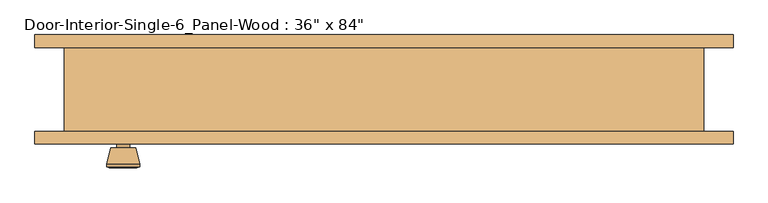
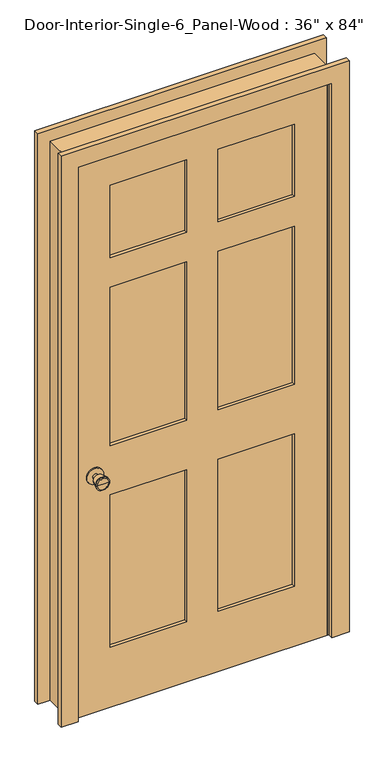
"""IFC4 building model written with IfcOpenShell, lengths in millimetres: door geometry."""

from ifc_helpers import new_model, si_unit, point, frame, frame_2d, origin, place, context, project, spatial, polyline, circle_curve, trimmed, segment, composite_curve, outline, extrude, faceted_brep, source, transform, mapped, element, save
from ifc_brep_helpers import plane_surface, cylinder_surface, revolved_surface, advanced_brep


def door_c610b25b(model_context):
    return source(origin(), model_context, "Body", "SolidModel", [
        advanced_brep(
        [(-393.7, -19.4, 914.4), (-403.7, -19.4, 914.4), (-383.7, -19.4, 914.4), (-373.2241324, 29.6, 914.4), (-414.1758676, 29.6, 914.4), (-393.7, 29.6, 914.4), (-368.7, 27.7721319, 914.4), (-418.7, 27.7721319, 914.4), (-368.7, 24.3084537, 914.4), (-418.7, 24.3084537, 914.4), (-375.063764, -0.4, 914.4), (-412.336236, -0.4, 914.4), (-383.7, -0.4, 914.4), (-403.7, -0.4, 914.4)],
        [
            (0, 1),
            (1, 2, circle_curve(frame((-393.7, -19.4, 914.4), z_axis=(0.0, -1.0, 0.0), x_axis=(-1.0, 0.0, 0.0)), 10.0)),
            (2, 0),
            (2, 1, circle_curve(frame((-393.7, -19.4, 914.4), z_axis=(0.0, -1.0, 0.0), x_axis=(-1.0, 0.0, 0.0)), 10.0)),
            (3, 4, circle_curve(frame((-393.7, 29.6, 914.4), z_axis=(0.0, 1.0, 0.0), x_axis=(-1.0, 0.0, 0.0)), 20.4758676)),
            (4, 5),
            (5, 3),
            (4, 3, circle_curve(frame((-393.7, 29.6, 914.4), z_axis=(0.0, 1.0, 0.0), x_axis=(-1.0, 0.0, 0.0)), 20.4758676)),
            (6, 7, circle_curve(frame((-393.7, 27.7721319, 914.4), z_axis=(0.0, 1.0, 0.0), x_axis=(-1.0, 0.0, 0.0)), 25.0)),
            (7, 4),
            (3, 6),
            (7, 6, circle_curve(frame((-393.7, 27.7721319, 914.4), z_axis=(0.0, 1.0, 0.0), x_axis=(-1.0, 0.0, 0.0)), 25.0)),
            (8, 9, circle_curve(frame((-393.7, 24.3084537, 914.4), z_axis=(0.0, 1.0, 0.0), x_axis=(-1.0, 0.0, 0.0)), 25.0)),
            (9, 7),
            (6, 8),
            (9, 8, circle_curve(frame((-393.7, 24.3084537, 914.4), z_axis=(0.0, 1.0, 0.0), x_axis=(-1.0, 0.0, 0.0)), 25.0)),
            (10, 11, circle_curve(frame((-393.7, -0.4, 914.4), z_axis=(0.0, 1.0, 0.0), x_axis=(-1.0, 0.0, 0.0)), 18.636236)),
            (11, 9),
            (8, 10),
            (11, 10, circle_curve(frame((-393.7, -0.4, 914.4), z_axis=(0.0, 1.0, 0.0), x_axis=(-1.0, 0.0, 0.0)), 18.636236)),
            (12, 13, circle_curve(frame((-393.7, -0.4, 914.4), z_axis=(0.0, 1.0, 0.0), x_axis=(-1.0, 0.0, 0.0)), 10.0)),
            (13, 11),
            (10, 12),
            (13, 12, circle_curve(frame((-393.7, -0.4, 914.4), z_axis=(0.0, 1.0, 0.0), x_axis=(-1.0, 0.0, 0.0)), 10.0)),
            (1, 13),
            (12, 2),
        ],
        [
            plane_surface(frame((-393.7, -19.4, 914.4), z_axis=(0.0, -1.0, 0.0), x_axis=(-1.0, 0.0, 0.0))),
            plane_surface(frame((-393.7, 29.6, 914.4), z_axis=(0.0, 1.0, 0.0), x_axis=(-1.0, 0.0, 0.0))),
            revolved_surface(polyline([(-414.1758676, 29.6, 914.4), (-418.7, 27.7721319, 914.4)]), (-393.7, -19.4, 914.4), (0.0, -1.0, 0.0)),
            cylinder_surface(frame((-393.7, -19.4, 914.4), z_axis=(0.0, -1.0, 0.0), x_axis=(-1.0, 0.0, 0.0)), 25.0),
            revolved_surface(polyline([(-418.7, 24.3084537, 914.4), (-412.336236, -0.4, 914.4)]), (-393.7, -19.4, 914.4), (0.0, -1.0, 0.0)),
            plane_surface(frame((-393.7, -0.4, 914.4), z_axis=(0.0, -1.0, 0.0), x_axis=(-1.0, 0.0, 0.0))),
            cylinder_surface(frame((-393.7, -19.4, 914.4), z_axis=(0.0, -1.0, 0.0), x_axis=(-1.0, 0.0, 0.0)), 10.0),
        ],
        [
            (0, [[1, 2, 3]]),
            (0, [[-3, 4, -1]]),
            (1, [[5, 6, 7]]),
            (1, [[8, -7, -6]]),
            (2, [[9, 10, -5, 11]]),
            (2, [[12, -11, -8, -10]]),
            (3, [[13, 14, -9, 15]]),
            (3, [[16, -15, -12, -14]]),
            (4, [[17, 18, -13, 19]]),
            (4, [[20, -19, -16, -18]]),
            (5, [[21, 22, -17, 23]]),
            (5, [[24, -23, -20, -22]]),
            (6, [[-2, 25, -21, 26]]),
            (6, [[-4, -26, -24, -25]]),
        ],
    ),
        extrude(outline(composite_curve([segment(trimmed(circle_curve(frame_2d((914.4, -393.7)), 30.0), [point((914.4, -423.7))], [point((914.4, -363.7))], False, "CARTESIAN"), True, "CONTINUOUS"), segment(trimmed(circle_curve(frame_2d((914.4, -393.7)), 30.0), [point((914.4, -363.7))], [point((914.4, -423.7))], False, "CARTESIAN"), True, "CONTINUOUS")], self_intersect=False)), frame((0.0, -25.4, 0.0), z_axis=(0.0, 1.0, 0.0), x_axis=(0.0, 0.0, 1.0)), (0.0, 0.0, 1.0), 6.0),
        advanced_brep(
        [(-393.7, -66.325, 914.4), (-383.7, -66.325, 914.4), (-403.7, -66.325, 914.4), (-373.2241324, -115.325, 914.4), (-393.7, -115.325, 914.4), (-414.1758676, -115.325, 914.4), (-368.7, -113.4971319, 914.4), (-418.7, -113.4971319, 914.4), (-368.7, -110.0334537, 914.4), (-418.7, -110.0334537, 914.4), (-375.063764, -85.325, 914.4), (-412.336236, -85.325, 914.4), (-383.7, -85.325, 914.4), (-403.7, -85.325, 914.4)],
        [
            (0, 1),
            (1, 2, circle_curve(frame((-393.7, -66.325, 914.4), z_axis=(0.0, 1.0, 0.0), x_axis=(-1.0, 0.0, 0.0)), 10.0)),
            (2, 0),
            (2, 1, circle_curve(frame((-393.7, -66.325, 914.4), z_axis=(0.0, 1.0, 0.0), x_axis=(-1.0, 0.0, 0.0)), 10.0)),
            (3, 4),
            (4, 5),
            (5, 3, circle_curve(frame((-393.7, -115.325, 914.4), z_axis=(0.0, -1.0, 0.0), x_axis=(-1.0, 0.0, 0.0)), 20.4758676)),
            (3, 5, circle_curve(frame((-393.7, -115.325, 914.4), z_axis=(0.0, -1.0, 0.0), x_axis=(-1.0, 0.0, 0.0)), 20.4758676)),
            (6, 3),
            (5, 7),
            (7, 6, circle_curve(frame((-393.7, -113.4971319, 914.4), z_axis=(0.0, -1.0, 0.0), x_axis=(-1.0, 0.0, 0.0)), 25.0)),
            (6, 7, circle_curve(frame((-393.7, -113.4971319, 914.4), z_axis=(0.0, -1.0, 0.0), x_axis=(-1.0, 0.0, 0.0)), 25.0)),
            (8, 6),
            (7, 9),
            (9, 8, circle_curve(frame((-393.7, -110.0334537, 914.4), z_axis=(0.0, -1.0, 0.0), x_axis=(-1.0, 0.0, 0.0)), 25.0)),
            (8, 9, circle_curve(frame((-393.7, -110.0334537, 914.4), z_axis=(0.0, -1.0, 0.0), x_axis=(-1.0, 0.0, 0.0)), 25.0)),
            (10, 8),
            (9, 11),
            (11, 10, circle_curve(frame((-393.7, -85.325, 914.4), z_axis=(0.0, -1.0, 0.0), x_axis=(-1.0, 0.0, 0.0)), 18.636236)),
            (10, 11, circle_curve(frame((-393.7, -85.325, 914.4), z_axis=(0.0, -1.0, 0.0), x_axis=(-1.0, 0.0, 0.0)), 18.636236)),
            (12, 10),
            (11, 13),
            (13, 12, circle_curve(frame((-393.7, -85.325, 914.4), z_axis=(0.0, -1.0, 0.0), x_axis=(-1.0, 0.0, 0.0)), 10.0)),
            (12, 13, circle_curve(frame((-393.7, -85.325, 914.4), z_axis=(0.0, -1.0, 0.0), x_axis=(-1.0, 0.0, 0.0)), 10.0)),
            (1, 12),
            (13, 2),
        ],
        [
            plane_surface(frame((-393.7, -66.325, 914.4), z_axis=(0.0, 1.0, 0.0), x_axis=(-1.0, 0.0, 0.0))),
            plane_surface(frame((-393.7, -115.325, 914.4), z_axis=(0.0, -1.0, 0.0), x_axis=(-1.0, 0.0, 0.0))),
            revolved_surface(polyline([(-414.1758676, -115.325, 914.4), (-418.7, -113.4971319, 914.4)]), (-393.7, -66.325, 914.4), (0.0, 1.0, 0.0)),
            cylinder_surface(frame((-393.7, -66.325, 914.4), z_axis=(0.0, 1.0, 0.0), x_axis=(-1.0, 0.0, 0.0)), 25.0),
            revolved_surface(polyline([(-418.7, -110.0334537, 914.4), (-412.336236, -85.325, 914.4)]), (-393.7, -66.325, 914.4), (0.0, 1.0, 0.0)),
            plane_surface(frame((-393.7, -85.325, 914.4), z_axis=(0.0, 1.0, 0.0), x_axis=(-1.0, 0.0, 0.0))),
            cylinder_surface(frame((-393.7, -66.325, 914.4), z_axis=(0.0, 1.0, 0.0), x_axis=(-1.0, 0.0, 0.0)), 10.0),
        ],
        [
            (0, [[1, 2, 3]]),
            (0, [[-3, 4, -1]]),
            (1, [[5, 6, 7]]),
            (1, [[-6, -5, 8]]),
            (2, [[9, -7, 10, 11]]),
            (2, [[-10, -8, -9, 12]]),
            (3, [[13, -11, 14, 15]]),
            (3, [[-14, -12, -13, 16]]),
            (4, [[17, -15, 18, 19]]),
            (4, [[-18, -16, -17, 20]]),
            (5, [[21, -19, 22, 23]]),
            (5, [[-22, -20, -21, 24]]),
            (6, [[25, -23, 26, -2]]),
            (6, [[-26, -24, -25, -4]]),
        ],
    ),
        extrude(outline(composite_curve([segment(trimmed(circle_curve(frame_2d((914.4, -393.7)), 30.0), [point((914.4, -423.7))], [point((914.4, -363.7))], False, "CARTESIAN"), True, "CONTINUOUS"), segment(trimmed(circle_curve(frame_2d((914.4, -393.7)), 30.0), [point((914.4, -363.7))], [point((914.4, -423.7))], False, "CARTESIAN"), True, "CONTINUOUS")], self_intersect=False)), frame((0.0, -66.325, 0.0), z_axis=(0.0, 1.0, 0.0), x_axis=(0.0, 0.0, 1.0)), (0.0, 0.0, 1.0), 6.0),
        faceted_brep([(482.6, -60.325, 0.0), (457.2, -60.325, 0.0), (457.2, -25.4, 0.0), (444.5, -25.4, 0.0), (444.5, 9.525, 0.0), (457.2, 9.525, 0.0), (457.2, 66.675, 0.0), (482.6, 66.675, 0.0), (482.6, 66.675, 2159.0), (482.6, -60.325, 2159.0), (457.2, 66.675, 2133.6), (-457.2, 66.675, 2133.6), (-457.2, 66.675, 0.0), (-482.6, 66.675, 0.0), (-482.6, 66.675, 2159.0), (457.2, 9.525, 2133.6), (444.5, 9.525, 2120.9), (-444.5, 9.525, 2120.9), (-444.5, 9.525, 0.0), (-457.2, 9.525, 0.0), (-457.2, 9.525, 2133.6), (444.5, -25.4, 2120.9), (457.2, -25.4, 2133.6), (-457.2, -25.4, 2133.6), (-457.2, -25.4, 0.0), (-444.5, -25.4, 0.0), (-444.5, -25.4, 2120.9), (457.2, -60.325, 2133.6), (-482.6, -60.325, 2159.0), (-482.6, -60.325, 0.0), (-457.2, -60.325, 0.0), (-457.2, -60.325, 2133.6)], [[[0, 1, 2, 3, 4, 5, 6, 7]], [[7, 8, 9, 0]], [[6, 10, 11, 12, 13, 14, 8, 7]], [[5, 15, 10, 6]], [[4, 16, 17, 18, 19, 20, 15, 5]], [[3, 21, 16, 4]], [[2, 22, 23, 24, 25, 26, 21, 3]], [[1, 27, 22, 2]], [[0, 9, 28, 29, 30, 31, 27, 1]], [[8, 14, 28, 9]], [[15, 20, 11, 10]], [[21, 26, 17, 16]], [[27, 31, 23, 22]], [[29, 13, 12, 19, 18, 25, 24, 30]], [[14, 13, 29, 28]], [[20, 19, 12, 11]], [[26, 25, 18, 17]], [[31, 30, 24, 23]]]),
        extrude(outline(polyline([(2133.6, -457.2), (0.0, -457.2), (0.0, 457.2), (2133.6, 457.2), (2133.6, -457.2)]), holes=[polyline([(2014.5375, 57.15), (2014.5375, 336.55), (1735.1375, 336.55), (1735.1375, 57.15), (2014.5375, 57.15)]), polyline([(1620.8375, 336.55), (1009.65, 336.55), (1009.65, 57.15), (1620.8375, 57.15), (1620.8375, 336.55)]), polyline([(1009.65, -57.15), (1009.65, -336.55), (1620.8375, -336.55), (1620.8375, -57.15), (1009.65, -57.15)]), polyline([(1735.1375, -336.55), (2014.5375, -336.55), (2014.5375, -57.15), (1735.1375, -57.15), (1735.1375, -336.55)]), polyline([(819.15, 57.15), (819.15, 336.55), (231.775, 336.55), (231.775, 57.15), (819.15, 57.15)]), polyline([(231.775, -57.15), (231.775, -336.55), (819.15, -336.55), (819.15, -57.15), (231.775, -57.15)])]), frame((0.0, -60.325, 0.0), z_axis=(0.0, 1.0, 0.0), x_axis=(0.0, 0.0, 1.0)), (0.0, 0.0, 1.0), 34.925),
        extrude(outline(polyline([(336.55, -37.0416667), (336.55, -48.6833333), (57.15, -48.6833333), (57.15, -37.0416667), (336.55, -37.0416667)])), frame((0.0, 0.0, 1735.1375), z_axis=(0.0, 0.0, 1.0), x_axis=(1.0, 0.0, 0.0)), (0.0, 0.0, 1.0), 279.4),
        extrude(outline(polyline([(336.55, -37.0416667), (336.55, -48.6833333), (57.15, -48.6833333), (57.15, -37.0416667), (336.55, -37.0416667)])), frame((0.0, 0.0, 1009.65), z_axis=(0.0, 0.0, 1.0), x_axis=(1.0, 0.0, 0.0)), (0.0, 0.0, 1.0), 611.1875),
        extrude(outline(polyline([(-57.15, -37.0416667), (-57.15, -48.6833333), (-336.55, -48.6833333), (-336.55, -37.0416667), (-57.15, -37.0416667)])), frame((0.0, 0.0, 1009.65), z_axis=(0.0, 0.0, 1.0), x_axis=(1.0, 0.0, 0.0)), (0.0, 0.0, 1.0), 611.1875),
        extrude(outline(polyline([(-57.15, -37.0416667), (-57.15, -48.6833333), (-336.55, -48.6833333), (-336.55, -37.0416667), (-57.15, -37.0416667)])), frame((0.0, 0.0, 1735.1375), z_axis=(0.0, 0.0, 1.0), x_axis=(1.0, 0.0, 0.0)), (0.0, 0.0, 1.0), 279.4),
        extrude(outline(polyline([(336.55, -37.0416667), (336.55, -48.6833333), (57.15, -48.6833333), (57.15, -37.0416667), (336.55, -37.0416667)])), frame((0.0, 0.0, 231.775), z_axis=(0.0, 0.0, 1.0), x_axis=(1.0, 0.0, 0.0)), (0.0, 0.0, 1.0), 587.375),
        extrude(outline(polyline([(-57.15, -37.0416667), (-57.15, -48.6833333), (-336.55, -48.6833333), (-336.55, -37.0416667), (-57.15, -37.0416667)])), frame((0.0, 0.0, 231.775), z_axis=(0.0, 0.0, 1.0), x_axis=(1.0, 0.0, 0.0)), (0.0, 0.0, 1.0), 587.375),
        extrude(outline(polyline([(0.0, 527.05), (2203.45, 527.05), (2203.45, -527.05), (0.0, -527.05), (0.0, -463.55), (2139.95, -463.55), (2139.95, 463.55), (0.0, 463.55), (0.0, 527.05)])), frame((0.0, -79.375, 0.0), z_axis=(0.0, 1.0, 0.0), x_axis=(0.0, 0.0, 1.0)), (0.0, 0.0, 1.0), 19.05),
        extrude(outline(polyline([(0.0, 527.05), (2203.45, 527.05), (2203.45, -527.05), (0.0, -527.05), (0.0, -463.55), (2139.95, -463.55), (2139.95, 463.55), (0.0, 463.55), (0.0, 527.05)])), frame((0.0, 66.675, 0.0), z_axis=(0.0, 1.0, 0.0), x_axis=(0.0, 0.0, 1.0)), (0.0, 0.0, 1.0), 19.05),
    ])


if __name__ == "__main__":
    model = new_model("IFC4")
    model_context = context("Model", 3, world=origin())
    ifc_project = project(units=[si_unit("LENGTHUNIT", "METRE", prefix="MILLI")], contexts=[model_context])
    site = spatial("IfcSite", under=ifc_project)
    building = spatial("IfcBuilding", under=site)
    placement = place(None, origin())
    door_shape = door_c610b25b(model_context)
    element("IfcDoor", 1, ObjectType="Door-Interior-Single-6_Panel-Wood : 36\" x 84\"", at=placement, inside=building, context=model_context, shape_type="MappedRepresentation", body=[
        mapped(door_shape, transform((0.0, 0.0, 0.0), x_axis=(1.0, 0.0, 0.0), y_axis=(0.0, 1.0, 0.0), z_axis=(0.0, 0.0, 1.0))),
    ])
    save(model, "model.ifc")

# Revit data of these elements
# Type "Door-Interior-Single-6_Panel-Wood : 36\" x 84\""
#   Type Mark = "10"
#   Assembly Code = "C1020300"
#   Analytic Construction = "Wooden"
#   Top Rail = 0' - 4 11/16"
#   Top Panel = 0' - 11"
#   Thickness = 0' - 1 3/8"
#   Thermal Resistance (R) = 2.5876 (h·ft²·°F)/BTU
#   Swing Angle [instance default] = 90.00°
#   Stiles = 0' - 4 3/4"
#   Rough Width = 3' - 2"
#   Rough Height = 7' - 1"
#   Mullion = 0' - 4 1/2"
#   Lock Rail = 0' - 7 1/2"
#   Intermediate Rail = 0' - 4 1/2"
#   Height = 7' - 0"
#   Width = 3' - 0"
#   Heat Transfer Coefficient (U) = 0.3865 BTU/(h·ft²·°F)
#   Bottom Rail = 0' - 9 1/8"
#   Trim Material = Cherry
#   Panel Material = Cherry
#   Frame Material = Cherry
#   Door Handle Material = Aluminum
#   Visual Light Transmittance = 0
#   Solar Heat Gain Coefficient = 0
#   Wall Closure = (empty or 0)
#   Function = (empty or 0)
# Element 1 (IfcDoor, "Door-Interior-Single-6_Panel-Wood : 36\" x 84\"")
#   Materials on its faces: "Cherry", "Aluminum"
# Materials
#   "Cherry": class "Wood", colour RGB 226 177 128, transparency 0, Description = "Prunus Serotina", Cost = 0
#   "Aluminum": class "Metal", colour RGB 247 247 247, transparency 0, Description = "Aluminum 6061", Cost = 0
